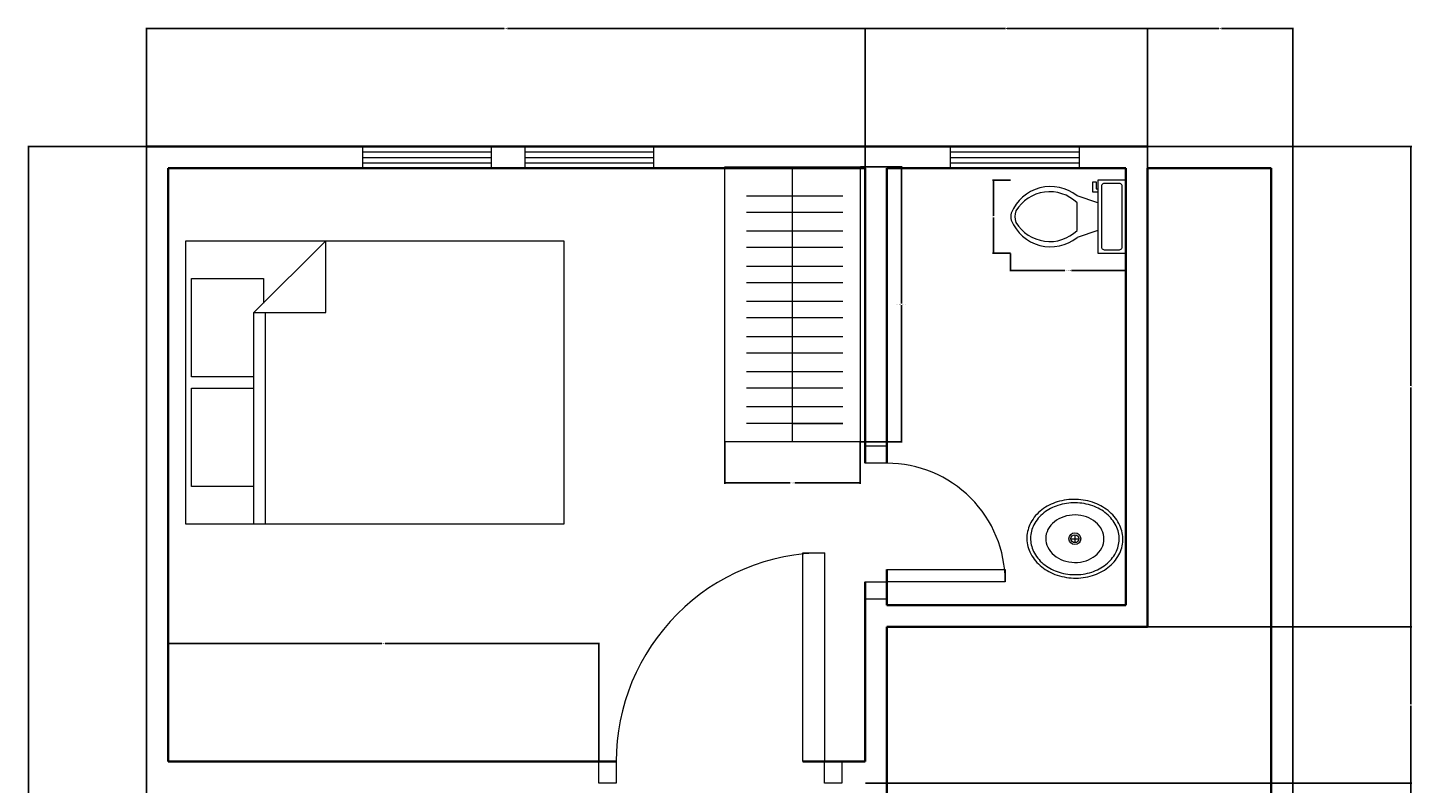
# Model space of a CAD drawing. Units: feet. Extents: x 2306 to 3052, y 829 to 1424.
# Tile 3 of 5: x 2306 to 2625, y 1250 to 1424. Entities that reach past the tile are written whole.
import ezdxf

# ---------------------------------------------------------------- set-up
doc = ezdxf.new("R2010")
doc.units = ezdxf.units.FT
for name, color, linetype, lineweight in [('A-ANNO-DIMS', 2, 'Continuous', 18), ('A-DOOR', 3, 'Continuous', 18), ('A-FLOR-FIXT', 9, 'Continuous', 18), ('A-FLOR-OTLN', 7, 'Continuous', 25), ('A-FURN', 8, 'Continuous', 13), ('A-GLAZ', 4, 'Continuous', 18), ('A-WALL', 7, 'Continuous', 35)]:
    doc.layers.add(name, color=color, linetype=linetype, lineweight=lineweight)
doc.styles.get("Standard").update_dxf_attribs({"font": 'arial.ttf'})
doc.dimstyles.get("Standard").update_dxf_attribs({"dimtxt": 0.18, "dimasz": 0.18, "dimexe": 0.18, "dimexo": 0.0625, "dimgap": 0.09, "dimtad": 0, "dimtih": 1, "dimtoh": 1, "dimdec": 4, "dimzin": 0, "dimdsep": 46, "dimlunit": 4, "dimtxsty": 'Standard', "dimcen": 0.09, "dimadec": 0, "dimazin": 0, "dimtfac": 1, "dimtdec": 4, "dimtofl": 0, "dimtmove": 0, "dimatfit": 3, "dimfxl": 1, "dimtolj": 1, "dimtzin": 0, "dimarcsym": 0})

# ---------------------------------------------------------------- blocks, each defined once
blk = doc.blocks.new('Window - Wood Frame 36 in. Wide plan')
for p, q in [((0, 6), (0, 0)), ((0, 4.5), (36, 4.5)), ((36, 6), (36, 0)), ((0, 3), (36, 3)), ((0, 1.5), (36, 1.5))]:
    blk.add_line(p, q)
blk = doc.blocks.new('Bed - Queen')
for p, q in [((0, -80.00003), (0, 0)), ((0, 0), (59.99999, 0)), ((59.99999, 0), (59.99999, -80.00003)), ((7.99999, -1.2), (28.79998, -1.2)), ((7.99999, -14.4), (7.99999, -1.2)), ((28.79998, -1.2), (28.79998, -14.4)), ((31.19999, -1.2), (51.99999, -1.2)), ((31.19999, -14.4), (31.19999, -1.2)), ((51.99999, -1.2), (51.99999, -16.4)), ((0, -14.4), (44.8, -14.4)), ((59.99999, -29.6), (44.8, -14.4)), ((44.8, -14.4), (44.8, -29.6)), ((44.8, -16.8), (0, -16.8)), ((51.99999, -16.4), (46.79936, -16.4)), ((44.8, -29.6), (59.99999, -29.6)), ((59.99999, -80.00003), (0, -80.00003))]:
    blk.add_line(p, q)
blk = doc.blocks.new('Toilet - top')
for p, q in [((9.5, -6), (9.5, -2)), ((-10, -8.5), (-8, -8.5)), ((-10, -9.5), (-10, -8.5)), ((-7, -9.5), (-10, -9.5)), ((-8, -8.5), (-8, -8)), ((-7, -8), (-7, -9.5)), ((-4, -8), (-6, -14)), ((4, -8), (6, -14)), ((4, -14), (-4, -14))]:
    blk.add_line(p, q)
blk.add_lwpolyline([(10.5, -8), (10.5, 0), (-10.5, 0), (-10.5, -8)], close=True)
for points in [[(-9.5, -2), (-9.5, -6)], [(8.5, -1), (-8.5, -1)], [(-8.5, -7), (8.5, -7)]]:
    blk.add_lwpolyline(points)
for centre, radius, start, end in [((-8.62, -1.88), 0.884, 81.8699, 188.1301), ((8.62, -1.88), 0.884, 351.8699, 98.1301), ((-8.62, -6.12), 0.884, 171.8699, 278.1301), ((8.62, -6.12), 0.884, 261.8699, 8.1301), ((3.52, -21.58), 12.17, 141.4691, 247.9714), ((4.2, -21.82), 11.33, 136.3677, 238.9468), ((-3.52, -21.58), 12.17, 292.0284, 38.5307), ((-4.2, -21.82), 11.33, 301.053, 43.6321), ((0, -27.88), 4, 245.7318, 294.2682), ((0, -29), 4, 254.8605, 285.1395)]:
    blk.add_arc(centre, radius, start, end)
blk = doc.blocks.new('Sink - Oval top')
for p, q in [((-1, 0), (1, 0)), ((0, 1), (0, -1))]:
    blk.add_line(p, q)
for points in [[(-12.23, 0.39, 0.117634), (-11.46, -3.36, 0.104469), (-8.88, -6.8, 0.090016), (-5.08, -9.07, 0.08192), (-0.32, -10.02, 0.08192), (4.49, -9.38, 0.090016), (8.42, -7.36, 0.104469), (11.22, -4.09, 0.117634), (12.23, -0.39, 0.117634), (11.46, 3.36, 0.104469), (8.88, 6.8, 0.090016), (5.08, 9.07, 0.08192), (0.32, 10.02, 0.08192), (-4.49, 9.38, 0.090016), (-8.42, 7.36, 0.104469), (-11.22, 4.09, 0.117634)], [(-11.29, 0.16, 0.118622), (-10.52, -3.25, 0.104678), (-8.07, -6.36, 0.089562), (-4.54, -8.37, 0.081185), (-0.13, -9.15, 0.081185), (4.3, -8.49, 0.089562), (7.89, -6.58, 0.104678), (10.42, -3.55, 0.118622), (11.29, -0.16, 0.118622), (10.52, 3.25, 0.104678), (8.07, 6.36, 0.089562), (4.54, 8.37, 0.081185), (0.13, 9.15, 0.081185), (-4.3, 8.49, 0.089562), (-7.89, 6.58, 0.104678), (-10.42, 3.55, 0.118622)], [(-7.42, 0.08, 0.118283), (-6.91, -2.17, 0.104607), (-5.29, -4.21, 0.089718), (-2.97, -5.53, 0.081436), (-0.07, -6.04, 0.081436), (2.84, -5.59, 0.089718), (5.2, -4.33, 0.104607), (6.86, -2.32, 0.118283), (7.42, -0.08, 0.118283), (6.91, 2.17, 0.104607), (5.29, 4.21, 0.089718), (2.97, 5.53, 0.081436), (0.07, 6.04, 0.081436), (-2.84, 5.59, 0.089718), (-5.2, 4.33, 0.104607), (-6.86, 2.32, 0.118283)]]:
    blk.add_lwpolyline(points, format="xyb", close=True)
for radius in [1.5, 1]:
    blk.add_circle((0, 0), radius)
blk = doc.blocks.new('DOOR-SWING-WIDE')
blk.add_lwpolyline([(52, 53), (52, 5), (56, 5), (56, 0), (52, 0), (52, 5), (47, 5), (47, 53), (48, 53), (52, 53, 0.414214), (4, 5)], format="xyb")
blk.add_lwpolyline([(4, 5), (4, 0), (0, 0), (0, 5)], close=True)
blk = doc.blocks.new('DOOR-SWING-STANDARD')
blk.add_lwpolyline([(4.02, 32.25), (4.02, 5), (1.75, 5)])
blk.add_lwpolyline([(4.02, 5), (6.86, 5), (6.86, 32.25), (6.29, 32.25), (4.02, 32.25, -0.414214), (31.27, 5)], format="xyb")
for points in [[(0, 5), (0, 0), (4, 0), (4, 5)], [(31.27, 5), (31.27, 0), (35.27, 0), (35.27, 5)]]:
    blk.add_lwpolyline(points, close=True)
blk = doc.blocks.new('WARDROBE-PLAN')
for p, q in [((0, 0), (0, 63.25)), ((0, 63.25), (8.03, 63.25)), ((2.89, 63.25), (31.17, 63.25)), ((15.59, 0), (15.59, 63.25)), ((31.17, 63.25), (31.17, 0)), ((27.14, 56.53), (4.98, 56.53)), ((27.14, 52.77), (4.98, 52.77)), ((27.14, 48.44), (4.98, 48.44)), ((27.14, 44.68), (4.98, 44.68)), ((27.14, 40.35), (4.98, 40.35)), ((27.14, 36.59), (4.98, 36.59)), ((27.14, 32.26), (4.98, 32.26)), ((27.14, 28.49), (4.98, 28.49)), ((27.14, 24.17), (4.98, 24.17)), ((27.14, 20.4), (4.98, 20.4)), ((27.14, 16.08), (4.98, 16.08)), ((27.14, 12.31), (4.98, 12.31)), ((27.14, 7.99), (4.98, 7.99)), ((27.14, 4.22), (4.98, 4.22)), ((15.59, 4.22), (27.14, 4.22)), ((31.17, 0), (0, 0))]:
    blk.add_line(p, q)
blk = doc.blocks.new('*D26')
at = {"layer": 'A-ANNO-DIMS', "color": 0, "lineweight": -2, "transparency": 16777216}
for p, q in [((2532.79, 1372.22), (2532.79, 1368.13)), ((2559.3, 1372.22), (2559.3, 1368.13)), ((2532.97, 1368.31), (2545.27, 1368.31)), ((2559.12, 1368.31), (2546.82, 1368.31))]:
    blk.add_line(p, q, dxfattribs=at)
at = {"layer": 'A-ANNO-DIMS', "color": 0, "transparency": 16777216}
for points in [[(2532.97, 1368.34), (2532.97, 1368.28), (2532.79, 1368.31)], [(2559.12, 1368.34), (2559.12, 1368.28), (2559.3, 1368.31)]]:
    blk.add_solid(points, dxfattribs=at)
at = {"layer": 'Defpoints', "color": 0, "transparency": 16777216}
for p in [(2532.79, 1372.28), (2559.3, 1372.28), (2559.3, 1368.31)]:
    blk.add_point(p, dxfattribs=at)
at = {"layer": 'A-ANNO-DIMS', "color": 0, "transparency": 16777216, "insert": (2546.05, 1368.31), "char_height": 0.18, "attachment_point": 5}
blk.add_mtext('\\A1;WC 27 TYP.', dxfattribs=at)
blk = doc.blocks.new('*D27')
at = {"layer": 'A-ANNO-DIMS', "color": 0, "lineweight": -2, "transparency": 16777216}
for p, q in [((2532.73, 1389.13), (2528.63, 1389.13)), ((2528.81, 1388.95), (2528.81, 1380.89)), ((2528.81, 1372.46), (2528.81, 1380.53)), ((2532.73, 1372.28), (2528.63, 1372.28))]:
    blk.add_line(p, q, dxfattribs=at)
at = {"layer": 'A-ANNO-DIMS', "color": 0, "transparency": 16777216}
for points in [[(2528.78, 1388.95), (2528.84, 1388.95), (2528.81, 1389.13)], [(2528.78, 1372.46), (2528.84, 1372.46), (2528.81, 1372.28)]]:
    blk.add_solid(points, dxfattribs=at)
at = {"layer": 'Defpoints', "color": 0, "transparency": 16777216}
for p in [(2532.79, 1389.13), (2528.81, 1372.28), (2532.79, 1372.28)]:
    blk.add_point(p, dxfattribs=at)
at = {"layer": 'A-ANNO-DIMS', "color": 0, "transparency": 16777216, "insert": (2528.81, 1380.71), "char_height": 0.18, "attachment_point": 5}
blk.add_mtext('\\A1;17 TYP.', dxfattribs=at)
blk = doc.blocks.new('*D30')
at = {"layer": 'A-ANNO-DIMS', "color": 0, "lineweight": -2, "transparency": 16777216}
for p, q in [((2498.21, 1392.17), (2507.82, 1392.17)), ((2507.64, 1391.99), (2507.64, 1360.73)), ((2507.64, 1329.1), (2507.64, 1360.36)), ((2498.21, 1328.92), (2507.82, 1328.92))]:
    blk.add_line(p, q, dxfattribs=at)
at = {"layer": 'A-ANNO-DIMS', "color": 0, "transparency": 16777216}
for points in [[(2507.61, 1391.99), (2507.67, 1391.99), (2507.64, 1392.17)], [(2507.61, 1329.1), (2507.67, 1329.1), (2507.64, 1328.92)]]:
    blk.add_solid(points, dxfattribs=at)
at = {"layer": 'Defpoints', "color": 0, "transparency": 16777216}
for p in [(2498.15, 1392.17), (2507.64, 1392.17), (2498.15, 1328.92)]:
    blk.add_point(p, dxfattribs=at)
at = {"layer": 'A-ANNO-DIMS', "color": 0, "transparency": 16777216, "insert": (2507.64, 1360.55), "char_height": 0.18, "attachment_point": 5}
blk.add_mtext('\\A1;WARDROBE 63 TYP.', dxfattribs=at)
blk = doc.blocks.new('*D31')
at = {"layer": 'A-ANNO-DIMS', "color": 0, "lineweight": -2, "transparency": 16777216}
for p, q in [((2466.98, 1328.86), (2466.98, 1319.25)), ((2498.15, 1328.86), (2498.15, 1319.25)), ((2467.16, 1319.43), (2482.04, 1319.43)), ((2497.97, 1319.43), (2483.09, 1319.43))]:
    blk.add_line(p, q, dxfattribs=at)
at = {"layer": 'A-ANNO-DIMS', "color": 0, "transparency": 16777216}
for points in [[(2467.16, 1319.46), (2467.16, 1319.4), (2466.98, 1319.43)], [(2497.97, 1319.46), (2497.97, 1319.4), (2498.15, 1319.43)]]:
    blk.add_solid(points, dxfattribs=at)
at = {"layer": 'Defpoints', "color": 0, "transparency": 16777216}
for p in [(2466.98, 1328.92), (2498.15, 1328.92), (2498.15, 1319.43)]:
    blk.add_point(p, dxfattribs=at)
at = {"layer": 'A-ANNO-DIMS', "color": 0, "transparency": 16777216, "insert": (2482.56, 1319.43), "char_height": 0.18, "attachment_point": 5}
blk.add_mtext('\\A1;31 TYP.', dxfattribs=at)
blk = doc.blocks.new('*D47')
at = {"layer": 'A-ANNO-DIMS', "color": 0, "lineweight": -2, "transparency": 16777216}
for p, q in [((2333.74, 1396.83), (2306.45, 1396.83)), ((2306.63, 1396.65), (2306.63, 1127.01)), ((2306.63, 857.01), (2306.63, 1126.65)), ((2333.74, 856.83), (2306.45, 856.83))]:
    blk.add_line(p, q, dxfattribs=at)
at = {"layer": 'A-ANNO-DIMS', "color": 0, "transparency": 16777216}
for points in [[(2306.6, 1396.65), (2306.66, 1396.65), (2306.63, 1396.83)], [(2306.6, 857.01), (2306.66, 857.01), (2306.63, 856.83)]]:
    blk.add_solid(points, dxfattribs=at)
at = {"layer": 'Defpoints', "color": 0, "transparency": 16777216}
for p in [(2306.63, 1396.83), (2333.8, 1396.83), (2333.8, 856.83)]:
    blk.add_point(p, dxfattribs=at)
at = {"layer": 'A-ANNO-DIMS', "color": 0, "transparency": 16777216, "insert": (2306.63, 1126.83), "char_height": 0.18, "attachment_point": 5}
blk.add_mtext('\\A1;540', dxfattribs=at)
blk = doc.blocks.new('*D51')
at = {"layer": 'A-ANNO-DIMS', "color": 0, "lineweight": -2, "transparency": 16777216}
for p, q in [((2499.37, 1250.33), (2625.16, 1250.33)), ((2624.98, 1250.15), (2624.98, 1220.51)), ((2624.98, 1190.51), (2624.98, 1220.15)), ((2592.87, 1190.33), (2625.16, 1190.33))]:
    blk.add_line(p, q, dxfattribs=at)
at = {"layer": 'A-ANNO-DIMS', "color": 0, "transparency": 16777216}
for points in [[(2624.95, 1250.15), (2625.01, 1250.15), (2624.98, 1250.33)], [(2624.95, 1190.51), (2625.01, 1190.51), (2624.98, 1190.33)]]:
    blk.add_solid(points, dxfattribs=at)
at = {"layer": 'Defpoints', "color": 0, "transparency": 16777216}
for p in [(2499.3, 1250.33), (2624.98, 1250.33), (2592.8, 1190.33)]:
    blk.add_point(p, dxfattribs=at)
at = {"layer": 'A-ANNO-DIMS', "color": 0, "transparency": 16777216, "insert": (2624.98, 1220.33), "char_height": 0.18, "attachment_point": 5}
blk.add_mtext('\\A1;60', dxfattribs=at)
blk = doc.blocks.new('*D52')
at = {"layer": 'A-ANNO-DIMS', "color": 0, "lineweight": -2, "transparency": 16777216}
for p, q in [((2564.37, 1286.33), (2625.16, 1286.33)), ((2624.98, 1286.15), (2624.98, 1268.51)), ((2624.98, 1250.51), (2624.98, 1268.15)), ((2499.37, 1250.33), (2625.16, 1250.33))]:
    blk.add_line(p, q, dxfattribs=at)
at = {"layer": 'A-ANNO-DIMS', "color": 0, "transparency": 16777216}
for points in [[(2624.95, 1286.15), (2625.01, 1286.15), (2624.98, 1286.33)], [(2624.95, 1250.51), (2625.01, 1250.51), (2624.98, 1250.33)]]:
    blk.add_solid(points, dxfattribs=at)
at = {"layer": 'Defpoints', "color": 0, "transparency": 16777216}
for p in [(2564.3, 1286.33), (2624.98, 1286.33), (2499.3, 1250.33)]:
    blk.add_point(p, dxfattribs=at)
at = {"layer": 'A-ANNO-DIMS', "color": 0, "transparency": 16777216, "insert": (2624.98, 1268.33), "char_height": 0.18, "attachment_point": 5}
blk.add_mtext('\\A1;36', dxfattribs=at)
blk = doc.blocks.new('*D53')
at = {"layer": 'A-ANNO-DIMS', "color": 0, "lineweight": -2, "transparency": 16777216}
for p, q in [((2597.87, 1396.83), (2625.16, 1396.83)), ((2624.98, 1396.65), (2624.98, 1341.76)), ((2624.98, 1286.51), (2624.98, 1341.4)), ((2564.37, 1286.33), (2625.16, 1286.33))]:
    blk.add_line(p, q, dxfattribs=at)
at = {"layer": 'A-ANNO-DIMS', "color": 0, "transparency": 16777216}
for points in [[(2624.95, 1396.65), (2625.01, 1396.65), (2624.98, 1396.83)], [(2624.95, 1286.51), (2625.01, 1286.51), (2624.98, 1286.33)]]:
    blk.add_solid(points, dxfattribs=at)
at = {"layer": 'Defpoints', "color": 0, "transparency": 16777216}
for p in [(2597.8, 1396.83), (2624.98, 1396.83), (2564.3, 1286.33)]:
    blk.add_point(p, dxfattribs=at)
at = {"layer": 'A-ANNO-DIMS', "color": 0, "transparency": 16777216, "insert": (2624.98, 1341.58), "char_height": 0.18, "attachment_point": 5}
blk.add_mtext('\\A1;110.5', dxfattribs=at)
blk = doc.blocks.new('*D54')
at = {"layer": 'A-ANNO-DIMS', "color": 0, "lineweight": -2, "transparency": 16777216}
for p, q in [((2333.8, 1396.89), (2333.8, 1424.18)), ((2333.98, 1424), (2416.17, 1424)), ((2499.12, 1424), (2416.94, 1424)), ((2499.3, 1391.89), (2499.3, 1424.18))]:
    blk.add_line(p, q, dxfattribs=at)
at = {"layer": 'A-ANNO-DIMS', "color": 0, "transparency": 16777216}
for points in [[(2333.98, 1424.03), (2333.98, 1423.97), (2333.8, 1424)], [(2499.12, 1424.03), (2499.12, 1423.97), (2499.3, 1424)]]:
    blk.add_solid(points, dxfattribs=at)
at = {"layer": 'Defpoints', "color": 0, "transparency": 16777216}
for p in [(2499.3, 1424), (2333.8, 1396.83), (2499.3, 1391.83)]:
    blk.add_point(p, dxfattribs=at)
at = {"layer": 'A-ANNO-DIMS', "color": 0, "transparency": 16777216, "insert": (2416.55, 1424), "char_height": 0.18, "attachment_point": 5}
blk.add_mtext('\\A1;165.5', dxfattribs=at)
blk = doc.blocks.new('*D55')
at = {"layer": 'A-ANNO-DIMS', "color": 0, "lineweight": -2, "transparency": 16777216}
for p, q in [((2499.3, 1391.89), (2499.3, 1424.18)), ((2499.48, 1424), (2531.58, 1424)), ((2564.12, 1424), (2532.02, 1424)), ((2564.3, 1391.89), (2564.3, 1424.18))]:
    blk.add_line(p, q, dxfattribs=at)
at = {"layer": 'A-ANNO-DIMS', "color": 0, "transparency": 16777216}
for points in [[(2499.48, 1424.03), (2499.48, 1423.97), (2499.3, 1424)], [(2564.12, 1424.03), (2564.12, 1423.97), (2564.3, 1424)]]:
    blk.add_solid(points, dxfattribs=at)
at = {"layer": 'Defpoints', "color": 0, "transparency": 16777216}
for p in [(2564.3, 1424), (2499.3, 1391.83), (2564.3, 1391.83)]:
    blk.add_point(p, dxfattribs=at)
at = {"layer": 'A-ANNO-DIMS', "color": 0, "transparency": 16777216, "insert": (2531.8, 1424), "char_height": 0.18, "attachment_point": 5}
blk.add_mtext('\\A1;65', dxfattribs=at)
blk = doc.blocks.new('*D56')
at = {"layer": 'A-ANNO-DIMS', "color": 0, "lineweight": -2, "transparency": 16777216}
for p, q in [((2564.3, 1391.89), (2564.3, 1424.18)), ((2564.48, 1424), (2580.73, 1424)), ((2597.62, 1424), (2581.38, 1424)), ((2597.8, 1396.89), (2597.8, 1424.18))]:
    blk.add_line(p, q, dxfattribs=at)
at = {"layer": 'A-ANNO-DIMS', "color": 0, "transparency": 16777216}
for points in [[(2564.48, 1424.03), (2564.48, 1423.97), (2564.3, 1424)], [(2597.62, 1424.03), (2597.62, 1423.97), (2597.8, 1424)]]:
    blk.add_solid(points, dxfattribs=at)
at = {"layer": 'Defpoints', "color": 0, "transparency": 16777216}
for p in [(2597.8, 1424), (2597.8, 1396.83), (2564.3, 1391.83)]:
    blk.add_point(p, dxfattribs=at)
at = {"layer": 'A-ANNO-DIMS', "color": 0, "transparency": 16777216, "insert": (2581.05, 1424), "char_height": 0.18, "attachment_point": 5}
blk.add_mtext('\\A1;33.5', dxfattribs=at)
blk = doc.blocks.new('*D59')
at = {"layer": 'A-ANNO-DIMS', "color": 0, "lineweight": -2, "transparency": 16777216}
for p, q in [((2338.8, 1255.39), (2338.8, 1282.68)), ((2338.98, 1282.5), (2387.98, 1282.5)), ((2437.76, 1282.5), (2388.76, 1282.5)), ((2437.94, 1255.39), (2437.94, 1282.68))]:
    blk.add_line(p, q, dxfattribs=at)
at = {"layer": 'A-ANNO-DIMS', "color": 0, "transparency": 16777216}
for points in [[(2338.98, 1282.53), (2338.98, 1282.47), (2338.8, 1282.5)], [(2437.76, 1282.53), (2437.76, 1282.47), (2437.94, 1282.5)]]:
    blk.add_solid(points, dxfattribs=at)
at = {"layer": 'Defpoints', "color": 0, "transparency": 16777216}
for p in [(2437.94, 1282.5), (2338.8, 1255.33), (2437.94, 1255.33)]:
    blk.add_point(p, dxfattribs=at)
at = {"layer": 'A-ANNO-DIMS', "color": 0, "transparency": 16777216, "insert": (2388.37, 1282.5), "char_height": 0.18, "attachment_point": 5}
blk.add_mtext('\\A1;99.13', dxfattribs=at)

msp = doc.modelspace()

# ---------------------------------------------------------------- linework, layer by layer
at = {"layer": 'A-DOOR'}
msp.add_lwpolyline([(2499.303, 1292.699), (2499.303, 1296.699)], dxfattribs=at)
at = {"layer": 'A-FLOR-OTLN'}
for p, q in [((2597.803, 1396.827), (2333.803, 1396.827)), ((2333.803, 1396.827), (2333.803, 856.827)), ((2597.803, 856.827), (2597.803, 1396.827))]:
    msp.add_line(p, q, dxfattribs=at)
at = {"layer": 'A-WALL'}
for p, q in [((2333.803, 1396.827), (2501.803, 1396.827)), ((2333.803, 1396.827), (2338.803, 1396.827)), ((2499.303, 1396.827), (2504.303, 1396.827)), ((2501.803, 1396.827), (2561.803, 1396.827)), ((2559.303, 1396.827), (2564.303, 1396.827)), ((2338.803, 1391.827), (2338.803, 1255.327)), ((2338.803, 1391.827), (2499.303, 1391.827)), ((2499.303, 1391.827), (2338.803, 1391.827)), ((2499.303, 1391.827), (2499.303, 1323.953)), ((2504.303, 1391.827), (2504.303, 1323.953)), ((2504.303, 1391.827), (2559.303, 1391.827)), ((2559.303, 1391.827), (2504.303, 1391.827)), ((2559.303, 1391.827), (2559.303, 1291.327)), ((2564.303, 1391.827), (2564.303, 1291.327)), ((2592.803, 1391.827), (2564.303, 1391.827)), ((2592.803, 1291.327), (2592.803, 1391.827)), ((2504.303, 1299.538), (2504.303, 1291.327)), ((2499.303, 1296.682), (2499.303, 1255.327)), ((2504.303, 1291.327), (2559.303, 1291.327)), ((2564.303, 1291.327), (2564.303, 1286.327)), ((2592.803, 1291.327), (2592.803, 1286.327)), ((2504.303, 1286.327), (2504.303, 1195.327)), ((2504.303, 1286.327), (2559.303, 1286.327)), ((2559.303, 1286.327), (2564.303, 1286.327)), ((2592.803, 1195.327), (2592.803, 1286.327)), ((2338.803, 1255.327), (2441.935, 1255.327)), ((2484.935, 1255.327), (2499.303, 1255.327))]:
    msp.add_line(p, q, dxfattribs=at)

# ---------------------------------------------------------------- block references
at = {"layer": 'A-DOOR', "extrusion": (0, 0, -1), "zscale": -1, "rotation": 89.99999999999763}
msp.add_blockref('DOOR-SWING-STANDARD', (-2499.303, 1292.683), dxfattribs=at)
at = {"layer": 'A-DOOR'}
msp.add_blockref('DOOR-SWING-WIDE', (2437.935, 1250.327), dxfattribs=at)
at = {"layer": 'A-FLOR-FIXT', "xscale": 0.8023769030949434, "yscale": 0.8023769030949434, "zscale": 0.8023769030949434, "rotation": 270}
msp.add_blockref('Toilet - top', (2559.303, 1380.709), dxfattribs=at)
at = {"layer": 'A-FLOR-FIXT', "xscale": 0.9036611704051442, "yscale": 0.9036611704051442, "zscale": 0.9036611704051442}
msp.add_blockref('Sink - Oval top', (2547.577, 1306.602), dxfattribs=at)
at = {"layer": 'A-FURN'}
msp.add_blockref('WARDROBE-PLAN', (2466.979, 1328.921), dxfattribs=at)
at = {"layer": 'A-FURN', "xscale": 1.087596012527482, "yscale": 1.087596012527482, "zscale": 1.087596012527482, "rotation": 90}
msp.add_blockref('Bed - Queen', (2342.854, 1309.924), dxfattribs=at)
at = {"layer": 'A-GLAZ', "xscale": 0.82338841385576, "yscale": 0.82338841385576, "zscale": 0.82338841385576}
for p in [(2383.509, 1391.887), (2420.924, 1391.887), (2518.89, 1391.887)]:
    msp.add_blockref('Window - Wood Frame 36 in. Wide plan', p, dxfattribs=at)

# ---------------------------------------------------------------- dimensions: what is measured, and where the dimension line sits
at = {"layer": 'A-ANNO-DIMS'}
for base, p1, p2, override, picture, middle in [((2499.303, 1424.002), (2333.803, 1396.827), (2499.303, 1391.827), {"dimdec": 1, "dimlfac": 1, "dimrnd": 0, "dimzin": 0, "dimdsep": 46, "dimlunit": 2}, '*D54', (2416.553, 1424.002)), ((2564.303, 1424.002), (2499.303, 1391.827), (2564.303, 1391.827), {"dimdec": 0, "dimlfac": 1, "dimrnd": 0, "dimzin": 0, "dimdsep": 46, "dimlunit": 2}, '*D55', (2531.803, 1424.002)), ((2597.803, 1424.002), (2564.303, 1391.827), (2597.803, 1396.827), {"dimdec": 1, "dimlfac": 1, "dimrnd": 0, "dimzin": 0, "dimdsep": 46, "dimlunit": 2}, '*D56', (2581.053, 1424.002))]:
    dim = msp.add_linear_dim(base=base, p1=p1, p2=p2, dimstyle='Standard', override=override, dxfattribs=at)
    dim.commit()
    dim.dimension.update_dxf_attribs({"geometry": picture, "text_midpoint": middle})
for base, p1, p2, angle, override, picture, middle in [((2306.628, 1396.827), (2333.803, 856.827), (2333.803, 1396.827), 90, {"dimdec": 0, "dimlfac": 1, "dimrnd": 0, "dimzin": 0, "dimdsep": 46, "dimlunit": 2}, '*D47', (2306.628, 1126.827)), ((2624.978, 1396.827), (2564.303, 1286.327), (2597.803, 1396.827), 90, {"dimdec": 1, "dimlfac": 1, "dimrnd": 0, "dimzin": 0, "dimdsep": 46, "dimlunit": 2}, '*D53', (2624.978, 1341.577)), ((2624.978, 1286.327), (2499.303, 1250.327), (2564.303, 1286.327), 90, {"dimdec": 0, "dimlfac": 1, "dimrnd": 0, "dimzin": 0, "dimdsep": 46, "dimlunit": 2}, '*D52', (2624.978, 1268.327)), ((2437.935, 1282.502), (2338.803, 1255.327), (2437.935, 1255.327), 0, {"dimdec": 2, "dimlfac": 1, "dimrnd": 0, "dimzin": 0, "dimdsep": 46, "dimlunit": 2}, '*D59', (2388.369, 1282.502)), ((2624.978, 1250.327), (2592.803, 1190.327), (2499.303, 1250.327), 90, {"dimdec": 0, "dimlfac": 1, "dimrnd": 0, "dimzin": 0, "dimdsep": 46, "dimlunit": 2}, '*D51', (2624.978, 1220.327))]:
    dim = msp.add_linear_dim(base=base, p1=p1, p2=p2, angle=angle, dimstyle='Standard', override=override, dxfattribs=at)
    dim.commit()
    dim.dimension.update_dxf_attribs({"geometry": picture, "text_midpoint": middle})
for base, p1, p2, angle, text, picture, middle in [((2507.637, 1392.174), (2498.149, 1328.921), (2498.149, 1392.174), 90, 'WARDROBE <> TYP.', '*D30', (2507.637, 1360.548)), ((2528.81, 1372.284), (2532.788, 1389.134), (2532.788, 1372.284), 270, '<> TYP.', '*D27', (2528.81, 1380.709))]:
    dim = msp.add_linear_dim(base=base, p1=p1, p2=p2, angle=angle, text=text, dimstyle='Standard', override={"dimdec": 0, "dimlfac": 1, "dimrnd": 0, "dimzin": 0, "dimdsep": 46, "dimlunit": 2}, dxfattribs=at)
    dim.commit()
    dim.dimension.update_dxf_attribs({"geometry": picture, "text_midpoint": middle})
for base, p1, p2, text, picture, middle in [((2559.303, 1368.307), (2532.788, 1372.284), (2559.303, 1372.284), 'WC <> TYP.', '*D26', (2546.045, 1368.307)), ((2498.149, 1319.433), (2466.979, 1328.921), (2498.149, 1328.921), '<> TYP.', '*D31', (2482.564, 1319.433))]:
    dim = msp.add_linear_dim(base=base, p1=p1, p2=p2, text=text, dimstyle='Standard', override={"dimdec": 0, "dimlfac": 1, "dimrnd": 0, "dimzin": 0, "dimdsep": 46, "dimlunit": 2}, dxfattribs=at)
    dim.commit()
    dim.dimension.update_dxf_attribs({"geometry": picture, "text_midpoint": middle})

doc.saveas('drawing.dxf')
